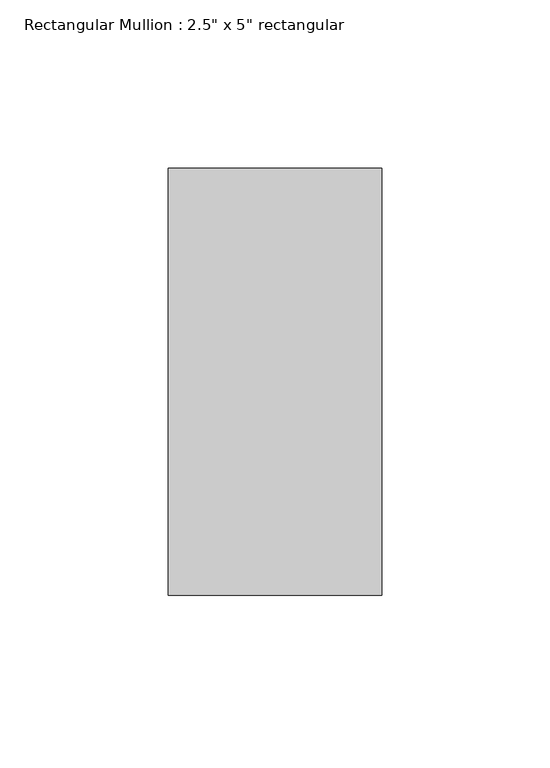
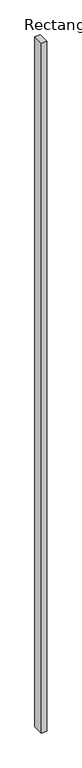
"""IFC4 building model written with IfcOpenShell, lengths in millimetres: member geometry."""

from ifc_helpers import new_model, si_unit, frame, origin, place, context, project, spatial, polyline, outline, extrude, source, transform, mapped, element, save


def member_6ded9322(model_context):
    return source(origin(), model_context, "Body", "SweptSolid", [
        extrude(outline(polyline([(0.0, 63.5), (0.0, -63.5), (-63.5, -63.5), (-63.5, 63.5), (0.0, 63.5)])), frame((0.0, 0.0, -8305.8349053), z_axis=(0.0, 0.0, 1.0), x_axis=(1.0, 0.0, 0.0)), (0.0, 0.0, 1.0), 8305.8349053),
    ])


if __name__ == "__main__":
    model = new_model("IFC4")
    model_context = context("Model", 3, world=origin())
    ifc_project = project(units=[si_unit("LENGTHUNIT", "METRE", prefix="MILLI")], contexts=[model_context])
    site = spatial("IfcSite", under=ifc_project)
    building = spatial("IfcBuilding", under=site)
    placement = place(None, origin())
    member_shape = member_6ded9322(model_context)
    element("IfcMember", 1, ObjectType="Rectangular Mullion : 2.5\" x 5\" rectangular", at=placement, inside=building, context=model_context, shape_type="MappedRepresentation", body=[
        mapped(member_shape, transform((0.0, 0.0, 0.0), x_axis=(1.0, 0.0, 0.0), y_axis=(0.0, 1.0, 0.0), z_axis=(0.0, 0.0, 1.0))),
    ])
    save(model, "model.ifc")

# Revit data of these elements
# Type "Rectangular Mullion : 2.5\" x 5\" rectangular"
#   built-in parameter 1007304 = 0.416667 (stored number, unit not read)
#   built-in parameter 1007301 = 0.104167 (stored number, unit not read)
#   built-in parameter 1007300 = 0.104167 (stored number, unit not read)
# Element 1 (IfcMember, "Rectangular Mullion : 2.5\" x 5\" rectangular")
#   Materials on its faces: "Aluminum"
# Materials
#   "Aluminum": class "Metal", colour RGB 247 247 247, transparency 0, Description = "Aluminum 6061", Cost = 0
